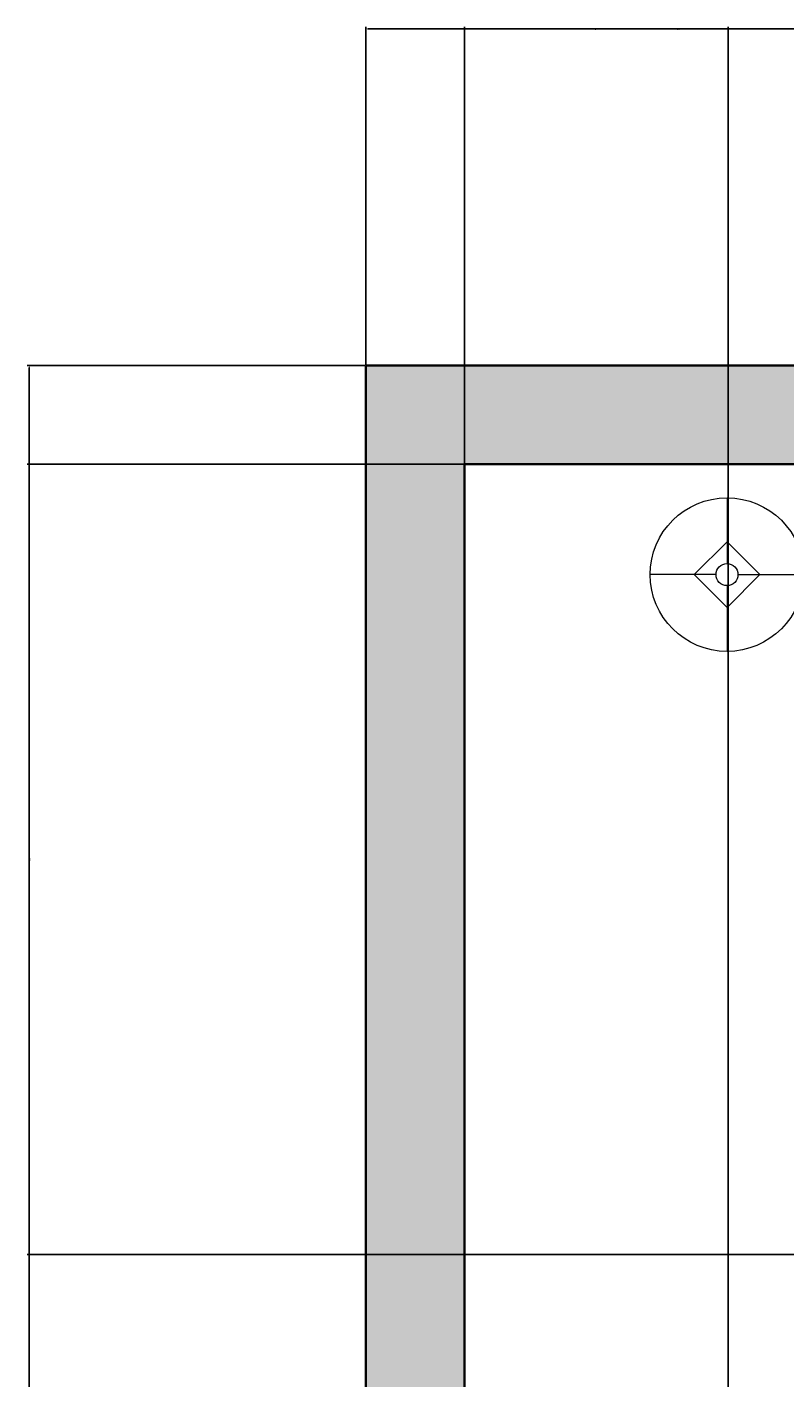
# Model space of a CAD drawing. Units: inches. Extents: x 1567 to 1964, y 1813 to 2447.
# Tile 14 of 28: x 1567 to 1636, y 2324 to 2447. Entities that reach past the tile are written whole.
import ezdxf

# ---------------------------------------------------------------- set-up
doc = ezdxf.new("R2010")
doc.units = ezdxf.units.IN
for name, color, linetype, lineweight in [('A-ANNO-DIMS', 2, 'Continuous', 18), ('A-FURN', 8, 'Continuous', 18), ('A-WALL', 7, 'Continuous', 35)]:
    doc.layers.add(name, color=color, linetype=linetype, lineweight=lineweight)
doc.layers.add('A-WALL-PATT', color=251, linetype='Continuous', lineweight=13, true_color=0x636466)
doc.styles.get("Standard").update_dxf_attribs({"font": 'arial.ttf'})
doc.dimstyles.get("Standard").update_dxf_attribs({"dimtxt": 0.18, "dimasz": 0.18, "dimexe": 0.18, "dimexo": 0.0625, "dimgap": 0.09, "dimtad": 0, "dimtih": 1, "dimtoh": 1, "dimdec": 4, "dimzin": 0, "dimdsep": 46, "dimtxsty": 'Standard', "dimcen": 0.09, "dimadec": 0, "dimazin": 0, "dimtfac": 1, "dimtdec": 4, "dimtofl": 0, "dimtmove": 0, "dimatfit": 3, "dimfxl": 1, "dimtolj": 1, "dimtzin": 0, "dimarcsym": 0})

# ---------------------------------------------------------------- blocks, each defined once
blk = doc.blocks.new('Lamp - Table')
for p, q in [((0, 7), (0, 1)), ((0, 3), (-3, 0)), ((3, 0), (0, 3)), ((-1, 0), (-7, 0)), ((-3, 0), (0, -3)), ((0, -3), (3, 0)), ((1, 0), (7, 0)), ((0, -1), (0, -7))]:
    blk.add_line(p, q)
for radius in [7, 1]:
    blk.add_circle((0, 0), radius)
blk = doc.blocks.new('*D41')
at = {"layer": 'A-ANNO-DIMS', "color": 0, "lineweight": -2, "transparency": 16777216}
for p, q in [((1597.37, 2416.29), (1566.6, 2416.29)), ((1566.78, 2416.11), (1566.78, 2160.47)), ((1566.78, 1904.47), (1566.78, 2160.11)), ((1601.37, 1904.29), (1566.6, 1904.29))]:
    blk.add_line(p, q, dxfattribs=at)
at = {"layer": 'A-ANNO-DIMS', "color": 0, "transparency": 16777216}
for points in [[(1566.75, 2416.11), (1566.81, 2416.11), (1566.78, 2416.29)], [(1566.75, 1904.47), (1566.81, 1904.47), (1566.78, 1904.29)]]:
    blk.add_solid(points, dxfattribs=at)
at = {"layer": 'Defpoints', "color": 0, "transparency": 16777216}
for p in [(1566.78, 2416.29), (1597.43, 2416.29), (1601.43, 1904.29)]:
    blk.add_point(p, dxfattribs=at)
at = {"layer": 'A-ANNO-DIMS', "color": 0, "transparency": 16777216, "insert": (1566.78, 2160.29), "char_height": 0.18, "attachment_point": 5}
blk.add_mtext('\\A1;512', dxfattribs=at)
blk = doc.blocks.new('*D43')
at = {"layer": 'A-ANNO-DIMS', "color": 0, "lineweight": -2, "transparency": 16777216}
for p, q in [((1597.43, 2416.35), (1597.43, 2447.12)), ((1597.61, 2446.94), (1625.71, 2446.94)), ((1654.25, 2446.94), (1626.15, 2446.94)), ((1654.43, 2416.35), (1654.43, 2447.12))]:
    blk.add_line(p, q, dxfattribs=at)
at = {"layer": 'A-ANNO-DIMS', "color": 0, "transparency": 16777216}
for points in [[(1597.61, 2446.97), (1597.61, 2446.91), (1597.43, 2446.94)], [(1654.25, 2446.97), (1654.25, 2446.91), (1654.43, 2446.94)]]:
    blk.add_solid(points, dxfattribs=at)
at = {"layer": 'Defpoints', "color": 0, "transparency": 16777216}
for p in [(1654.43, 2446.94), (1597.43, 2416.29), (1654.43, 2416.29)]:
    blk.add_point(p, dxfattribs=at)
at = {"layer": 'A-ANNO-DIMS', "color": 0, "transparency": 16777216, "insert": (1625.93, 2446.94), "char_height": 0.18, "attachment_point": 5}
blk.add_mtext('\\A1;57', dxfattribs=at)
blk = doc.blocks.new('*D48')
at = {"layer": 'A-ANNO-DIMS', "color": 0, "lineweight": -2, "transparency": 16777216}
for p, q in [((1742.37, 2407.29), (1566.6, 2407.29)), ((1566.78, 2407.11), (1566.78, 2371.47)), ((1566.78, 2335.47), (1566.78, 2371.11)), ((1742.37, 2335.29), (1566.6, 2335.29))]:
    blk.add_line(p, q, dxfattribs=at)
at = {"layer": 'A-ANNO-DIMS', "color": 0, "transparency": 16777216}
for points in [[(1566.75, 2407.11), (1566.81, 2407.11), (1566.78, 2407.29)], [(1566.75, 2335.47), (1566.81, 2335.47), (1566.78, 2335.29)]]:
    blk.add_solid(points, dxfattribs=at)
at = {"layer": 'Defpoints', "color": 0, "transparency": 16777216}
for p in [(1742.43, 2407.29), (1566.78, 2335.29), (1742.43, 2335.29)]:
    blk.add_point(p, dxfattribs=at)
at = {"layer": 'A-ANNO-DIMS', "color": 0, "transparency": 16777216, "insert": (1566.78, 2371.29), "char_height": 0.18, "attachment_point": 5}
blk.add_mtext('\\A1;72', dxfattribs=at)
blk = doc.blocks.new('*D53')
at = {"layer": 'A-ANNO-DIMS', "color": 0, "lineweight": -2, "transparency": 16777216}
for p, q in [((1606.43, 1913.35), (1606.43, 2447.12)), ((1606.61, 2446.94), (1618.21, 2446.94)), ((1630.25, 2446.94), (1618.65, 2446.94)), ((1630.43, 1913.35), (1630.43, 2447.12))]:
    blk.add_line(p, q, dxfattribs=at)
at = {"layer": 'A-ANNO-DIMS', "color": 0, "transparency": 16777216}
for points in [[(1606.61, 2446.97), (1606.61, 2446.91), (1606.43, 2446.94)], [(1630.25, 2446.97), (1630.25, 2446.91), (1630.43, 2446.94)]]:
    blk.add_solid(points, dxfattribs=at)
at = {"layer": 'Defpoints', "color": 0, "transparency": 16777216}
for p in [(1630.43, 2446.94), (1606.43, 1913.29), (1630.43, 1913.29)]:
    blk.add_point(p, dxfattribs=at)
at = {"layer": 'A-ANNO-DIMS', "color": 0, "transparency": 16777216, "insert": (1618.43, 2446.94), "char_height": 0.18, "attachment_point": 5}
blk.add_mtext('\\A1;24', dxfattribs=at)
blk = doc.blocks.new('*D56')
at = {"layer": 'A-ANNO-DIMS', "color": 0, "lineweight": -2, "transparency": 16777216}
for p, q in [((1606.43, 2127.35), (1606.43, 2447.12)), ((1606.61, 2446.94), (1618.21, 2446.94)), ((1630.25, 2446.94), (1618.65, 2446.94)), ((1630.43, 2127.35), (1630.43, 2447.12))]:
    blk.add_line(p, q, dxfattribs=at)
at = {"layer": 'A-ANNO-DIMS', "color": 0, "transparency": 16777216}
for points in [[(1606.61, 2446.97), (1606.61, 2446.91), (1606.43, 2446.94)], [(1630.25, 2446.97), (1630.25, 2446.91), (1630.43, 2446.94)]]:
    blk.add_solid(points, dxfattribs=at)
at = {"layer": 'Defpoints', "color": 0, "transparency": 16777216}
for p in [(1630.43, 2446.94), (1606.43, 2127.29), (1630.43, 2127.29)]:
    blk.add_point(p, dxfattribs=at)
at = {"layer": 'A-ANNO-DIMS', "color": 0, "transparency": 16777216, "insert": (1618.43, 2446.94), "char_height": 0.18, "attachment_point": 5}
blk.add_mtext('\\A1;24', dxfattribs=at)
blk = doc.blocks.new('*D57')
at = {"layer": 'A-ANNO-DIMS', "color": 0, "lineweight": -2, "transparency": 16777216}
for p, q in [((1630.43, 2127.35), (1630.43, 2447.12)), ((1630.61, 2446.94), (1654.21, 2446.94)), ((1678.25, 2446.94), (1654.65, 2446.94)), ((1678.43, 2127.35), (1678.43, 2447.12))]:
    blk.add_line(p, q, dxfattribs=at)
at = {"layer": 'A-ANNO-DIMS', "color": 0, "transparency": 16777216}
for points in [[(1630.61, 2446.97), (1630.61, 2446.91), (1630.43, 2446.94)], [(1678.25, 2446.97), (1678.25, 2446.91), (1678.43, 2446.94)]]:
    blk.add_solid(points, dxfattribs=at)
at = {"layer": 'Defpoints', "color": 0, "transparency": 16777216}
for p in [(1678.43, 2446.94), (1630.43, 2127.29), (1678.43, 2127.29)]:
    blk.add_point(p, dxfattribs=at)
at = {"layer": 'A-ANNO-DIMS', "color": 0, "transparency": 16777216, "insert": (1654.43, 2446.94), "char_height": 0.18, "attachment_point": 5}
blk.add_mtext('\\A1;48', dxfattribs=at)

msp = doc.modelspace()

# ---------------------------------------------------------------- hatches: boundary and pattern name
at = {"layer": 'A-WALL-PATT'}
h = msp.add_hatch(color=256, dxfattribs=at)
h.dxf.hatch_style = 1
h.paths.add_polyline_path([(1606.4295, 2407.29), (1654.4295, 2407.29), (1654.4295, 2416.29), (1597.4295, 2416.29), (1597.4295, 2217.29), (1606.4295, 2217.29), (1606.4295, 2259.29), (1738.4295, 2259.29), (1738.4295, 2247.29), (1742.4295, 2247.29), (1742.4295, 2259.29), (1742.4295, 2272.29), (1738.4295, 2272.29), (1738.4295, 2263.29), (1606.4295, 2263.29)])
h.paths.add_polyline_path([(1753.4295, 2416.29), (1690.4295, 2416.29), (1690.4295, 2407.29), (1738.4295, 2407.29), (1738.4295, 2308.29), (1742.4295, 2308.29), (1742.4295, 2331.29), (1746.9295, 2331.29), (1746.9295, 2335.29), (1742.4295, 2335.29), (1742.4295, 2407.29), (1753.4295, 2407.29)])
h.paths.add_polyline_path([(1840.4295, 2416.29), (1777.4295, 2416.29), (1777.4295, 2407.29), (1788.4295, 2407.29), (1788.4295, 2335.29), (1776.9295, 2335.29), (1776.9295, 2331.29), (1788.4295, 2331.29), (1788.4295, 2308.29), (1792.4295, 2308.29), (1792.4295, 2407.29), (1840.4295, 2407.29)])
h.paths.add_polyline_path([(1933.4295, 2416.29), (1876.4295, 2416.29), (1876.4295, 2407.29), (1924.4295, 2407.29), (1924.4295, 2263.29), (1792.4295, 2263.29), (1792.4295, 2272.29), (1788.4295, 2272.29), (1788.4295, 2259.29), (1872.4295, 2259.29), (1872.4295, 2171.29), (1880.9295, 2171.29), (1880.9295, 2175.29), (1876.4295, 2175.29), (1876.4295, 2259.29), (1924.4295, 2259.29), (1924.4295, 2229.29), (1933.4295, 2229.29)])
h.paths.add_polyline_path([(1933.4295, 2205.29), (1924.4295, 2205.29), (1924.4295, 2175.29), (1910.9295, 2175.29), (1910.9295, 2171.29), (1924.4295, 2171.29), (1924.4295, 2127.29), (1844.4295, 2127.29), (1844.4295, 2123.29), (1924.4295, 2123.29), (1924.4295, 2063.29), (1933.4295, 2063.29)])
h.paths.add_polyline_path([(1799.4295, 2123.29), (1808.4295, 2123.29), (1808.4295, 2127.29), (1781.4295, 2127.29), (1781.4295, 2123.29), (1795.4295, 2123.29), (1795.4295, 1964.29), (1711.4295, 1964.29), (1711.4295, 2123.29), (1751.4295, 2123.29), (1751.4295, 2127.29), (1742.4295, 2127.29), (1742.4295, 2139.29), (1738.4295, 2139.29), (1738.4295, 2127.29), (1678.4295, 2127.29), (1678.4295, 2123.29), (1702.4295, 2123.29), (1702.4295, 1913.29), (1678.4295, 1913.29), (1678.4295, 1904.29), (1711.4295, 1904.29), (1711.4295, 1960.29), (1795.4295, 1960.29), (1795.4295, 1906.69), (1929.4295, 1906.69), (1929.4295, 1848.29), (1601.4295, 1848.29), (1601.4295, 1904.29), (1630.4295, 1904.29), (1630.4295, 1913.29), (1606.4295, 1913.29), (1606.4295, 2123.29), (1630.4295, 2123.29), (1630.4295, 2127.29), (1606.4295, 2127.29), (1606.4295, 2169.29), (1597.4295, 2169.29), (1597.4295, 1844.29), (1933.4295, 1844.29), (1933.4295, 2027.29), (1924.4295, 2027.29), (1924.4295, 1967.29), (1833.9295, 1967.29), (1833.9295, 1963.29), (1924.4295, 1963.29), (1924.4295, 1910.69), (1799.4295, 1910.69), (1799.4295, 1963.29), (1803.9295, 1963.29), (1803.9295, 1967.29), (1799.4295, 1967.29)])

# ---------------------------------------------------------------- linework, layer by layer
at = {"layer": 'A-WALL'}
for p, q in [((1597.4295, 2416.29), (1933.4295, 2416.29)), ((1597.4295, 1844.29), (1597.4295, 2416.29)), ((1606.4295, 2407.29), (1738.4295, 2407.29)), ((1606.4295, 2263.29), (1606.4295, 2407.29))]:
    msp.add_line(p, q, dxfattribs=at)

# ---------------------------------------------------------------- block references
at = {"layer": 'A-FURN'}
msp.add_blockref('Lamp - Table', (1630.3402, 2397.2257), dxfattribs=at)

# ---------------------------------------------------------------- dimensions: what is measured, and where the dimension line sits
at = {"layer": 'A-ANNO-DIMS'}
for base, p1, p2, picture, middle in [((1654.4295, 2446.94), (1597.4295, 2416.29), (1654.4295, 2416.29), '*D43', (1625.9295, 2446.94)), ((1630.4295, 2446.94), (1606.4295, 1913.29), (1630.4295, 1913.29), '*D53', (1618.4295, 2446.94)), ((1630.4295, 2446.94), (1606.4295, 2127.29), (1630.4295, 2127.29), '*D56', (1618.4295, 2446.94)), ((1678.4295, 2446.94), (1630.4295, 2127.29), (1678.4295, 2127.29), '*D57', (1654.4295, 2446.94))]:
    dim = msp.add_linear_dim(base=base, p1=p1, p2=p2, dimstyle='Standard', override={"dimdec": 0, "dimlfac": 1, "dimrnd": 0, "dimzin": 0, "dimdsep": 46, "dimlunit": 2}, dxfattribs=at)
    dim.commit()
    dim.dimension.update_dxf_attribs({"geometry": picture, "text_midpoint": middle})
for base, p1, p2, picture, middle in [((1566.7795, 2416.29), (1601.4295, 1904.29), (1597.4295, 2416.29), '*D41', (1566.7795, 2160.29)), ((1566.7795, 2335.29), (1742.4295, 2407.29), (1742.4295, 2335.29), '*D48', (1566.7795, 2371.29))]:
    dim = msp.add_linear_dim(base=base, p1=p1, p2=p2, angle=90, dimstyle='Standard', override={"dimdec": 0, "dimlfac": 1, "dimrnd": 0, "dimzin": 0, "dimdsep": 46, "dimlunit": 2}, dxfattribs=at)
    dim.commit()
    dim.dimension.update_dxf_attribs({"geometry": picture, "text_midpoint": middle})

doc.saveas('drawing.dxf')
